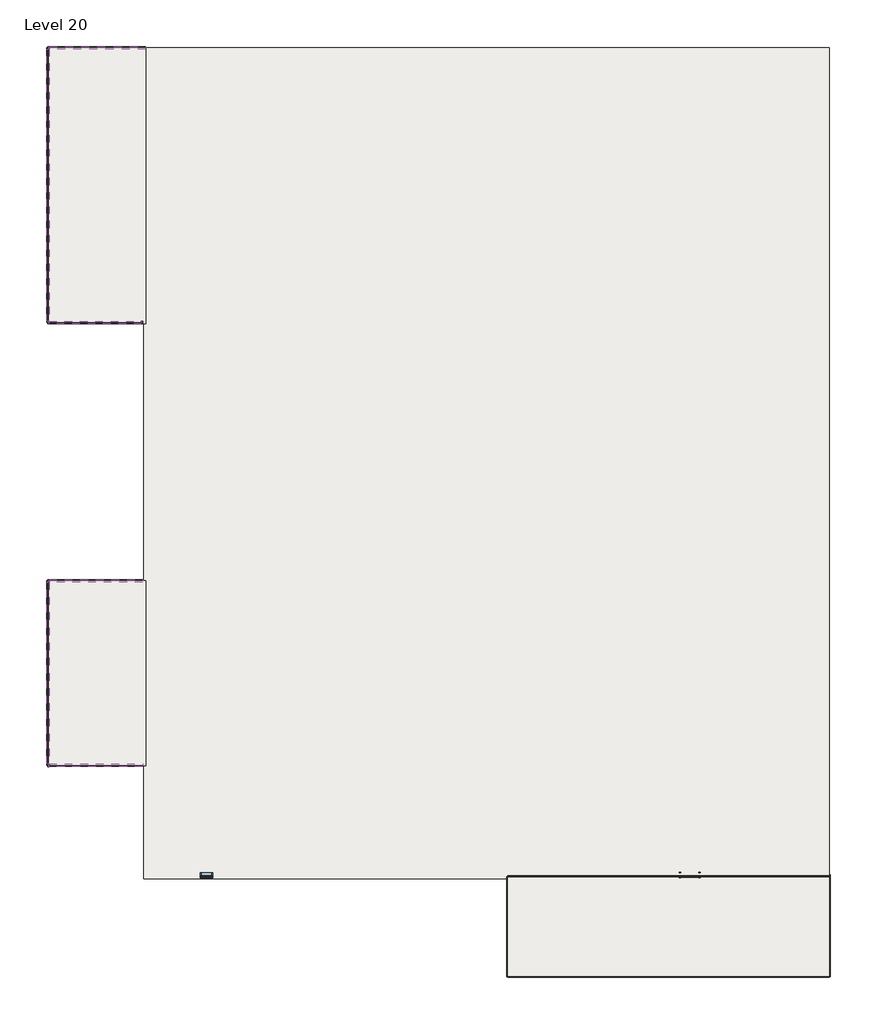
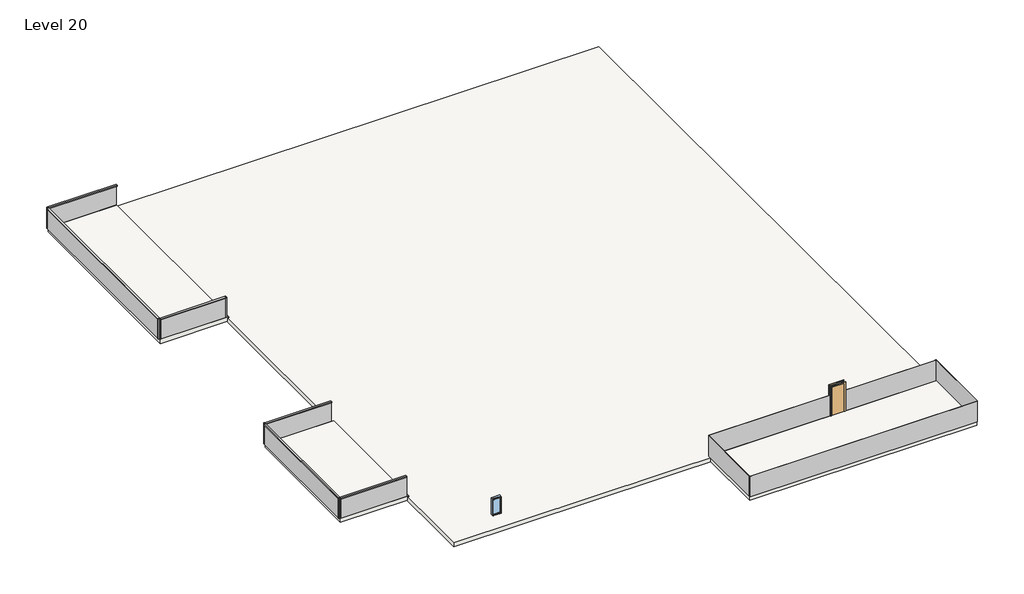
# One storey: 15 members, 10 plates, 4 slabs, 1 door, 1 window.
"""IFC4 building model written with IfcOpenShell, lengths in millimetres."""

from ifc_helpers import new_model, si_unit, frame, origin, place, context, project, spatial, polyline, outline, extrude, transform, mapped, element, save
from components import door_719f80de, member_4491d118, member_ab1dc975, member_e63cd10b, member_a7b860c5, member_01548017, member_4960e788, system_panel_glazed_dbf8c7ac, system_panel_glazed_79055968, system_panel_glazed_00b49b46, system_panel_glazed_e6f20943, system_panel_glazed_ba9ccfd0, system_panel_glazed_53b9e4d0, system_panel_glazed_0656cd8c, system_panel_glazed_1f6fd899, window_78885257

model = new_model("IFC4")

# Units and contexts
model_context = context("Model", 3, world=origin())
ifc_project = project(units=[si_unit("LENGTHUNIT", "METRE", prefix="MILLI")], contexts=[model_context])

# Site, building, storey
site = spatial("IfcSite", under=ifc_project)
building = spatial("IfcBuilding", under=site)
storey = spatial("IfcBuildingStorey", under=building, Name="Level 20", Elevation=32918.4)

# Door
placement = place(None, origin())
door_shape = door_719f80de(model_context)
element("IfcDoor", 1, ObjectType="Single-Flush : 36\" x 84\"", at=placement, inside=storey, context=model_context, shape_type="MappedRepresentation", body=[
    mapped(door_shape, transform((12155.361926, -20744.1985361, 32918.4), x_axis=(1.0, 0.0, 0.0), y_axis=(0.0, 1.0, 0.0), z_axis=(0.0, 0.0, 1.0))),
])

# Members
member_shape = member_4491d118(model_context)
element("IfcMember", 2, ObjectType="Rectangular Mullion : 2.5\" x 5\" rectangular", at=placement, inside=storey, context=model_context, shape_type="MappedRepresentation", body=[
    mapped(member_shape, transform((-20096.288074, 7013.3807139, 32918.4), x_axis=(-1.0, 0.0, 0.0), y_axis=(0.0, 1.0, 0.0), z_axis=(0.0, 0.0, -1.0))),
])
element("IfcMember", 3, ObjectType="Rectangular Mullion : 2.5\" x 5\" rectangular", at=placement, inside=storey, context=model_context, shape_type="MappedRepresentation", body=[
    mapped(member_shape, transform((-20096.288074, 20810.2014639, 32918.4), x_axis=(0.0, 1.0, 0.0), y_axis=(1.0, 0.0, 0.0), z_axis=(0.0, 0.0, -1.0))),
])
element("IfcMember", 4, ObjectType="Rectangular Mullion : 2.5\" x 5\" rectangular", at=placement, inside=storey, context=model_context, shape_type="MappedRepresentation", body=[
    mapped(member_shape, transform((-20096.288074, -5966.8213044, 32918.4), x_axis=(0.0, 1.0, 0.0), y_axis=(1.0, 0.0, 0.0), z_axis=(0.0, 0.0, -1.0))),
])
element("IfcMember", 5, ObjectType="Rectangular Mullion : 2.5\" x 5\" rectangular", at=placement, inside=storey, context=model_context, shape_type="MappedRepresentation", body=[
    mapped(member_shape, transform((-20096.288074, -15231.4713044, 32918.4), x_axis=(-1.0, 0.0, 0.0), y_axis=(0.0, 1.0, 0.0), z_axis=(0.0, 0.0, -1.0))),
])
member_2_shape = member_ab1dc975(model_context)
element("IfcMember", 6, ObjectType="Rectangular Mullion : 2.5\" x 5\" rectangular", at=placement, inside=storey, context=model_context, shape_type="MappedRepresentation", body=[
    mapped(member_2_shape, transform((-20032.788074, 7013.3807139, 34442.4), x_axis=(0.0, 0.0, 1.0), y_axis=(0.0, 1.0, 0.0), z_axis=(-1.0, 0.0, 0.0))),
])
element("IfcMember", 7, ObjectType="Rectangular Mullion : 2.5\" x 5\" rectangular", at=placement, inside=storey, context=model_context, shape_type="MappedRepresentation", body=[
    mapped(member_shape, transform((-20096.288074, 7013.3807139, 34442.4), x_axis=(0.0, -1.0, 0.0), y_axis=(1.0, 0.0, 0.0), z_axis=(0.0, 0.0, 1.0))),
])
element("IfcMember", 8, ObjectType="Rectangular Mullion : 2.5\" x 5\" rectangular", at=placement, inside=storey, context=model_context, shape_type="MappedRepresentation", body=[
    mapped(member_shape, transform((-15328.7800649, 7013.3807139, 34442.4), x_axis=(1.0, 0.0, 0.0), y_axis=(0.0, 1.0, 0.0), z_axis=(0.0, 0.0, 1.0))),
])
element("IfcMember", 9, ObjectType="Rectangular Mullion : 2.5\" x 5\" rectangular", at=placement, inside=storey, context=model_context, shape_type="MappedRepresentation", body=[
    mapped(member_shape, transform((-20096.288074, 20810.2014639, 34442.4), x_axis=(-1.0, 0.0, 0.0), y_axis=(0.0, -1.0, 0.0), z_axis=(0.0, 0.0, 1.0))),
])
element("IfcMember", 10, ObjectType="Rectangular Mullion : 2.5\" x 5\" rectangular", at=placement, inside=storey, context=model_context, shape_type="MappedRepresentation", body=[
    mapped(member_shape, transform((-20096.288074, -5966.8213044, 34442.4), x_axis=(-1.0, 0.0, 0.0), y_axis=(0.0, -1.0, 0.0), z_axis=(0.0, 0.0, 1.0))),
])
element("IfcMember", 11, ObjectType="Rectangular Mullion : 2.5\" x 5\" rectangular", at=placement, inside=storey, context=model_context, shape_type="MappedRepresentation", body=[
    mapped(member_shape, transform((-20096.288074, -15231.4713044, 34442.4), x_axis=(0.0, -1.0, 0.0), y_axis=(1.0, 0.0, 0.0), z_axis=(0.0, 0.0, 1.0))),
])
member_3_shape = member_e63cd10b(model_context)
element("IfcMember", 12, ObjectType="Rectangular Mullion : 2.5\" x 5\" rectangular", at=placement, inside=storey, context=model_context, shape_type="MappedRepresentation", body=[
    mapped(member_3_shape, transform((-15175.038074, 20810.2014639, 34442.4), x_axis=(0.0, 0.0, 1.0), y_axis=(0.0, -1.0, 0.0), z_axis=(1.0, 0.0, 0.0))),
])
member_4_shape = member_a7b860c5(model_context)
element("IfcMember", 13, ObjectType="Rectangular Mullion : 2.5\" x 5\" rectangular", at=placement, inside=storey, context=model_context, shape_type="MappedRepresentation", body=[
    mapped(member_4_shape, transform((-20096.288074, 20746.7014639, 34442.4), x_axis=(0.0, 0.0, 1.0), y_axis=(1.0, 0.0, 0.0), z_axis=(0.0, 1.0, 0.0))),
])
member_5_shape = member_01548017(model_context)
element("IfcMember", 14, ObjectType="Rectangular Mullion : 2.5\" x 5\" rectangular", at=placement, inside=storey, context=model_context, shape_type="MappedRepresentation", body=[
    mapped(member_5_shape, transform((-15333.788074, -5966.8213044, 34442.4), x_axis=(0.0, 0.0, 1.0), y_axis=(0.0, -1.0, 0.0), z_axis=(1.0, 0.0, 0.0))),
])
member_6_shape = member_4960e788(model_context)
element("IfcMember", 15, ObjectType="Rectangular Mullion : 2.5\" x 5\" rectangular", at=placement, inside=storey, context=model_context, shape_type="MappedRepresentation", body=[
    mapped(member_6_shape, transform((-20096.288074, -6030.3213044, 34442.4), x_axis=(0.0, 0.0, 1.0), y_axis=(1.0, 0.0, 0.0), z_axis=(0.0, 1.0, 0.0))),
])
element("IfcMember", 16, ObjectType="Rectangular Mullion : 2.5\" x 5\" rectangular", at=placement, inside=storey, context=model_context, shape_type="MappedRepresentation", body=[
    mapped(member_5_shape, transform((-20032.788074, -15231.4713044, 34442.4), x_axis=(0.0, 0.0, 1.0), y_axis=(0.0, 1.0, 0.0), z_axis=(-1.0, 0.0, 0.0))),
])

# Plates
system_panel_glazed_shape = system_panel_glazed_dbf8c7ac(model_context)
element("IfcPlate", 17, ObjectType="System Panel : Glazed", at=placement, inside=storey, context=model_context, shape_type="MappedRepresentation", body=[
    mapped(system_panel_glazed_shape, transform((11088.561926, -20824.2135805, 32918.4), x_axis=(1.0, 0.0, 0.0), y_axis=(0.0, 1.0, 0.0), z_axis=(0.0, 0.0, 1.0))),
])
element("IfcPlate", 18, ObjectType="System Panel : Glazed", at=placement, inside=storey, context=model_context, shape_type="MappedRepresentation", body=[
    mapped(system_panel_glazed_shape, transform((11088.561926, -25847.4170305, 32918.4), x_axis=(-1.0, 0.0, 0.0), y_axis=(0.0, -1.0, 0.0), z_axis=(0.0, 0.0, 1.0))),
])
system_panel_glazed_2_shape = system_panel_glazed_79055968(model_context)
element("IfcPlate", 19, ObjectType="System Panel : Glazed", at=placement, inside=storey, context=model_context, shape_type="MappedRepresentation", body=[
    mapped(system_panel_glazed_2_shape, transform((3011.361926, -23335.8153055, 32918.4), x_axis=(0.0, 1.0, 0.0), y_axis=(-1.0, 0.0, 0.0), z_axis=(0.0, 0.0, 1.0))),
])
system_panel_glazed_3_shape = system_panel_glazed_00b49b46(model_context)
element("IfcPlate", 20, ObjectType="System Panel : Glazed", at=placement, inside=storey, context=model_context, shape_type="MappedRepresentation", body=[
    mapped(system_panel_glazed_3_shape, transform((19165.761926, -23295.8077833, 32918.4), x_axis=(0.0, -1.0, 0.0), y_axis=(1.0, 0.0, 0.0), z_axis=(0.0, 0.0, 1.0))),
])
system_panel_glazed_4_shape = system_panel_glazed_e6f20943(model_context)
element("IfcPlate", 21, ObjectType="System Panel : Glazed", at=placement, inside=storey, context=model_context, shape_type="MappedRepresentation", body=[
    mapped(system_panel_glazed_4_shape, transform((-17712.5340694, 7013.3807139, 32918.4), x_axis=(-1.0, 0.0, 0.0), y_axis=(0.0, -1.0, 0.0), z_axis=(0.0, 0.0, 1.0))),
])
system_panel_glazed_5_shape = system_panel_glazed_ba9ccfd0(model_context)
element("IfcPlate", 22, ObjectType="System Panel : Glazed", at=placement, inside=storey, context=model_context, shape_type="MappedRepresentation", body=[
    mapped(system_panel_glazed_5_shape, transform((-17603.913074, 20810.2014639, 32918.4), x_axis=(1.0, 0.0, 0.0), y_axis=(0.0, 1.0, 0.0), z_axis=(0.0, 0.0, 1.0))),
])
system_panel_glazed_6_shape = system_panel_glazed_53b9e4d0(model_context)
element("IfcPlate", 23, ObjectType="System Panel : Glazed", at=placement, inside=storey, context=model_context, shape_type="MappedRepresentation", body=[
    mapped(system_panel_glazed_6_shape, transform((-20096.288074, 13911.7910889, 32918.4), x_axis=(0.0, 1.0, 0.0), y_axis=(-1.0, 0.0, 0.0), z_axis=(0.0, 0.0, 1.0))),
])
system_panel_glazed_7_shape = system_panel_glazed_0656cd8c(model_context)
element("IfcPlate", 24, ObjectType="System Panel : Glazed", at=placement, inside=storey, context=model_context, shape_type="MappedRepresentation", body=[
    mapped(system_panel_glazed_7_shape, transform((-17683.288074, -5966.8213044, 32918.4), x_axis=(1.0, 0.0, 0.0), y_axis=(0.0, 1.0, 0.0), z_axis=(0.0, 0.0, 1.0))),
])
element("IfcPlate", 25, ObjectType="System Panel : Glazed", at=placement, inside=storey, context=model_context, shape_type="MappedRepresentation", body=[
    mapped(system_panel_glazed_7_shape, transform((-17683.288074, -15231.4713044, 32918.4), x_axis=(-1.0, 0.0, 0.0), y_axis=(0.0, -1.0, 0.0), z_axis=(0.0, 0.0, 1.0))),
])
system_panel_glazed_8_shape = system_panel_glazed_1f6fd899(model_context)
element("IfcPlate", 26, ObjectType="System Panel : Glazed", at=placement, inside=storey, context=model_context, shape_type="MappedRepresentation", body=[
    mapped(system_panel_glazed_8_shape, transform((-20096.288074, -10599.1463044, 32918.4), x_axis=(0.0, 1.0, 0.0), y_axis=(-1.0, 0.0, 0.0), z_axis=(0.0, 0.0, 1.0))),
])

# Slabs
element("IfcSlab", 27, ObjectType="Generic - 12\"", at=placement, inside=storey, context=model_context, shape_type="SweptSolid", body=[
    extrude(outline(polyline([(19166.5126981, 20817.2004767), (19166.5126981, -20940.3995233), (-15275.8873019, -20940.3995233), (-15275.8873019, 20817.2004767), (19166.5126981, 20817.2004767)])), frame((0.0, 0.0, 32527.5835276), z_axis=(0.0, 0.0, 1.0), x_axis=(1.0, 0.0, 0.0)), (0.0, 0.0, 1.0), 304.8),
])
element("IfcSlab", 28, ObjectType="Generic - 12\"", at=placement, inside=storey, context=model_context, shape_type="SweptSolid", body=[
    extrude(outline(polyline([(3011.361926, -20845.7985361), (19165.761926, -20845.7985361), (19165.761926, -25828.3670305), (3011.361926, -25828.3670305), (3011.361926, -20845.7985361)])), frame((0.0, 0.0, 32613.6), z_axis=(0.0, 0.0, 1.0), x_axis=(1.0, 0.0, 0.0)), (0.0, 0.0, 1.0), 304.8),
])
element("IfcSlab", 29, ObjectType="Generic - 12\"", at=placement, inside=storey, context=model_context, shape_type="SweptSolid", body=[
    extrude(outline(polyline([(-20051.838074, -15263.2213044), (-20051.838074, -5966.8213044), (-15175.038074, -5966.8213044), (-15175.038074, -15263.2213044), (-20051.838074, -15263.2213044)])), frame((0.0, 0.0, 32613.6), z_axis=(0.0, 0.0, 1.0), x_axis=(1.0, 0.0, 0.0)), (0.0, 0.0, 1.0), 304.8),
])
element("IfcSlab", 30, ObjectType="Generic - 12\"", at=placement, inside=storey, context=model_context, shape_type="SweptSolid", body=[
    extrude(outline(polyline([(-20051.838074, 20810.2014639), (-15175.038074, 20810.2014639), (-15175.038074, 6941.8014639), (-20051.838074, 6941.8014639), (-20051.838074, 20810.2014639)])), frame((0.0, 0.0, 32613.6), z_axis=(0.0, 0.0, 1.0), x_axis=(1.0, 0.0, 0.0)), (0.0, 0.0, 1.0), 304.8),
])

# Window
window_shape = window_78885257(model_context)
element("IfcWindow", 31, ObjectType="Instance - Fixed : 24\" x 48\"", at=placement, inside=storey, context=model_context, shape_type="MappedRepresentation", body=[
    mapped(window_shape, transform((-12165.138074, -20744.1985361, 32918.4), x_axis=(-1.0, 0.0, 0.0), y_axis=(0.0, -1.0, 0.0), z_axis=(0.0, 0.0, 1.0))),
])

save(model, "model.ifc")

# Revit data of these elements
# Type "Single-Flush : 36\" x 84\""
#   Type Mark = "1"
#   Construction Type Id = "MDOOR"
#   Assembly Code = "C1020"
#   Analytic Construction = "Metal"
#   Thickness = 0' - 2"
#   Heat Transfer Coefficient (U) = 0.651978 BTU/(h·ft²·°F)
#   Height = 7' - 0"
#   Trim Projection Ext = 0' - 1"
#   Trim Projection Int = 0' - 1"
#   Trim Width = 0' - 3"
#   Width = 3' - 0"
#   Define Thermal Properties by = 1
#   Door Material = Door - Panel
#   Frame Material = Door - Frame
#   Visual Light Transmittance = 0
#   Solar Heat Gain Coefficient = 0
#   Function = (empty or 0)
#   Wall Closure = (empty or 0)
# Type "Rectangular Mullion : 2.5\" x 5\" rectangular"
#   built-in parameter 1007304 = 0.416667 (stored number, unit not read)
#   built-in parameter 1007301 = 0.104167 (stored number, unit not read)
#   built-in parameter 1007300 = 0.104167 (stored number, unit not read)
# Type "System Panel : Glazed"
#   Construction Type Id = "GSP4R"
#   Analytic Construction = "1/8 in Pilkington single glazing"
#   Visual Light Transmittance = 0.9
#   Solar Heat Gain Coefficient = 0.86
#   Heat Transfer Coefficient (U) = 1.18115 BTU/(h·ft²·°F)
# Type "Generic - 12\""
#   Assembly Code = "B1010"
#   Function = 0
#   Layers, outside or top first: 1' - 0" no material (function 1)
# Type "Instance - Fixed : 24\" x 48\""
#   Type Mark = "19"
#   Construction Type Id = "GSP4R"
#   Assembly Code = "B2020100"
#   Analytic Construction = "1/8 in Pilkington single glazing"
#   Visual Light Transmittance = 0.9
#   Thermal Resistance (R) = 0.8466 (h·ft²·°F)/BTU
#   Solar Heat Gain Coefficient = 0.86
#   Heat Transfer Coefficient (U) = 1.1812 BTU/(h·ft²·°F)
#   Height [instance default] = 4' - 0"
#   Default Sill Height = 3' - 0"
#   Width [instance default] = 2' - 0"
#   Window Inset = 0' - 0 3/4"
#   Define Thermal Properties by = 1
#   Glass Pane Material = Glass
#   Sash Material = Sash
#   Wall Closure = (empty or 0)
# Element 1 (IfcDoor, "Single-Flush : 36\" x 84\"")
#   Phase Created = New Construction
#   Materials on its faces: "Door - Frame", "Door - Panel"
# Elements 2, 3, 4, 5, 6, 7, 8, 9, 10, 11, 12, 13, 14, 15, 16 (IfcMember, "Rectangular Mullion : 2.5\" x 5\" rectangular")
#   Phase Created = New Construction
#   Materials on its faces: "Aluminum"
# Elements 17, 18, 19, 20, 21, 22, 23, 24, 25, 26 (IfcPlate, "System Panel : Glazed")
#   Phase Created = New Construction
#   Materials on its faces: "Glass"
# Element 27 (IfcSlab, "Generic - 12\"")
#   Height Offset From Level = -0' - 3.38648"
#   Phase Created = New Construction
#   Materials on its faces: "Default Floor"
# Elements 28, 29, 30 (IfcSlab, "Generic - 12\"")
#   built-in parameter 1001955 = 3.14159 (stored number, unit not read)
#   Height Offset From Level = 0' - 0"
#   Phase Created = New Construction
#   Materials on its faces: "Default Floor"
# Element 31 (IfcWindow, "Instance - Fixed : 24\" x 48\"")
#   Mark = "13"
#   Width = 2' - 0"
#   Height = 4' - 0"
#   Phase Created = New Construction
#   Materials on its faces: "Sash", "Glass"
# Materials
#   "Door - Panel": class "Wood", colour RGB 210 159 95, transparency 0
#   "Door - Frame": colour RGB 118 70 51, transparency 0
#   "Glass": class "Glass", colour RGB 0 128 192, transparency 0.75, Description = "Soda Lime Glass", Cost = 0
#   "Sash": class "Wood", colour RGB 224 178 126, transparency 0
#   "Aluminum": class "Metal", colour RGB 247 247 247, transparency 0, Description = "Aluminum 6061", Cost = 0
#   "Default Floor": colour RGB 128 128 128, transparency 0
